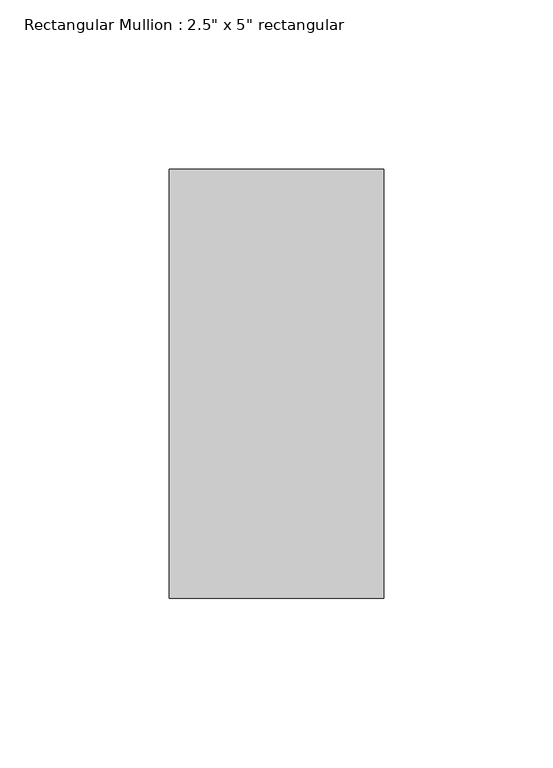
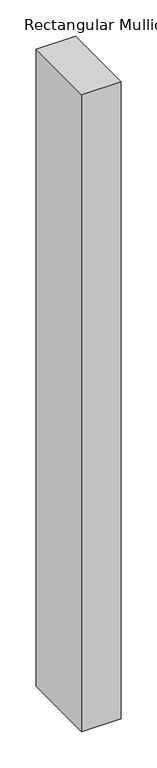
"""IFC4 building model written with IfcOpenShell, lengths in millimetres: member geometry."""

from ifc_helpers import new_model, si_unit, frame, origin, place, context, project, spatial, polyline, outline, extrude, source, transform, mapped, element, save


def member_bf0a6844(model_context):
    return source(origin(), model_context, "Body", "SweptSolid", [
        extrude(outline(polyline([(31.75, 63.5), (31.75, -63.5), (-31.75, -63.5), (-31.75, 63.5), (31.75, 63.5)])), frame((0.0, 0.0, -1079.5), z_axis=(0.0, 0.0, 1.0), x_axis=(1.0, 0.0, 0.0)), (0.0, 0.0, 1.0), 1079.5),
    ])


if __name__ == "__main__":
    model = new_model("IFC4")
    model_context = context("Model", 3, world=origin())
    ifc_project = project(units=[si_unit("LENGTHUNIT", "METRE", prefix="MILLI")], contexts=[model_context])
    site = spatial("IfcSite", under=ifc_project)
    building = spatial("IfcBuilding", under=site)
    placement = place(None, origin())
    member_shape = member_bf0a6844(model_context)
    element("IfcMember", 1, ObjectType="Rectangular Mullion : 2.5\" x 5\" rectangular", at=placement, inside=building, context=model_context, shape_type="MappedRepresentation", body=[
        mapped(member_shape, transform((0.0, 0.0, 0.0), x_axis=(1.0, 0.0, 0.0), y_axis=(0.0, 1.0, 0.0), z_axis=(0.0, 0.0, 1.0))),
    ])
    save(model, "model.ifc")

# Revit data of these elements
# Type "Rectangular Mullion : 2.5\" x 5\" rectangular"
#   built-in parameter 1007304 = 0.416667 (stored number, unit not read)
#   built-in parameter 1007301 = 0.104167 (stored number, unit not read)
#   built-in parameter 1007300 = 0.104167 (stored number, unit not read)
# Element 1 (IfcMember, "Rectangular Mullion : 2.5\" x 5\" rectangular")
#   Materials on its faces: "Aluminum"
# Materials
#   "Aluminum": class "Metal", colour RGB 247 247 247, transparency 0, Description = "Aluminum 6061", Cost = 0
